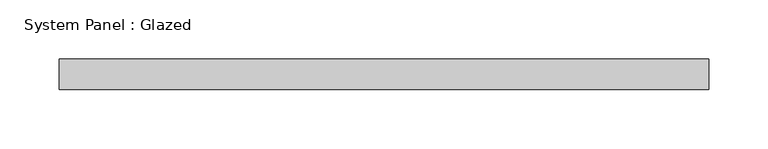
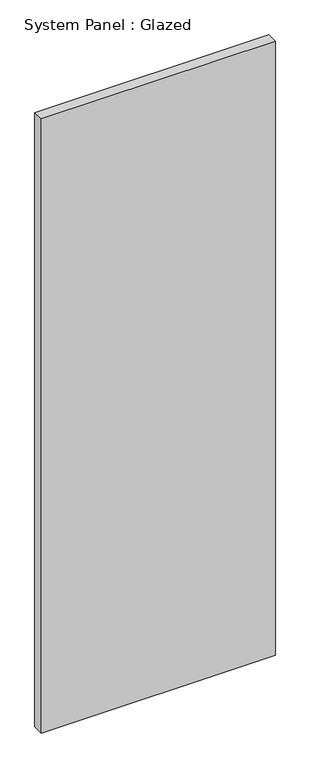
"""IFC4 building model written with IfcOpenShell, lengths in millimetres: plate geometry, System Panel : Glazed."""

from ifc_helpers import new_model, si_unit, origin, origin_with_axes, place, context, project, spatial, polyline, outline, extrude, source, transform, mapped, element, save


def system_panel_glazed_a2ae5ad6(model_context):
    return source(origin(), model_context, "Body", "SweptSolid", [
        extrude(outline(polyline([(273.05, 19.05), (-273.05, 19.05), (-273.05, 44.45), (273.05, 44.45), (273.05, 19.05)])), origin_with_axes(), (0.0, 0.0, 1.0), 1513.1839946),
    ])


if __name__ == "__main__":
    model = new_model("IFC4")
    model_context = context("Model", 3, world=origin())
    ifc_project = project(units=[si_unit("LENGTHUNIT", "METRE", prefix="MILLI")], contexts=[model_context])
    site = spatial("IfcSite", under=ifc_project)
    building = spatial("IfcBuilding", under=site)
    placement = place(None, origin())
    system_panel_glazed_shape = system_panel_glazed_a2ae5ad6(model_context)
    element("IfcPlate", 1, ObjectType="System Panel : Glazed", at=placement, inside=building, context=model_context, shape_type="MappedRepresentation", body=[
        mapped(system_panel_glazed_shape, transform((0.0, 0.0, 0.0), x_axis=(1.0, 0.0, 0.0), y_axis=(0.0, 1.0, 0.0), z_axis=(0.0, 0.0, 1.0))),
    ])
    save(model, "model.ifc")

# Revit data of these elements
# Type "System Panel : Glazed"
#   Construction Type Id = "GSP4R"
#   Analytic Construction = "1/8 in Pilkington single glazing"
#   Visual Light Transmittance = 0.9
#   Solar Heat Gain Coefficient = 0.86
#   Heat Transfer Coefficient (U) = 1.18115 BTU/(h·ft²·°F)
#   Define Thermal Properties by = 1
# Element 1 (IfcPlate, "System Panel : Glazed")
#   Materials on its faces: "Glass"
# Materials
#   "Glass": class "Glass", colour RGB 0 128 192, transparency 0.75, Description = "Soda Lime Glass", Cost = 0
